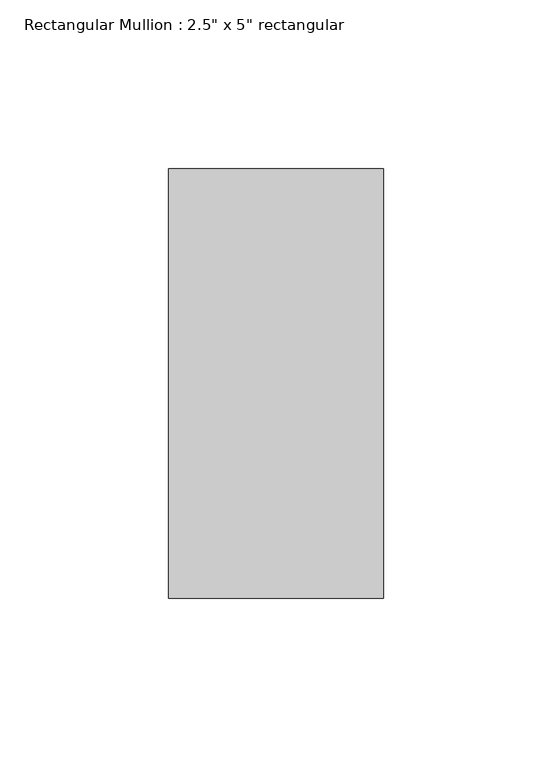
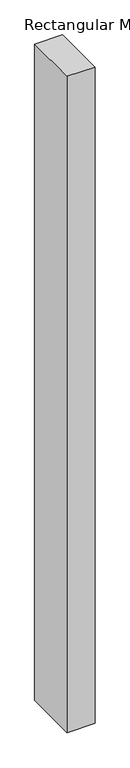
"""IFC4 building model written with IfcOpenShell, lengths in millimetres: member geometry."""

from ifc_helpers import new_model, si_unit, frame, origin, place, context, project, spatial, polyline, outline, extrude, source, transform, mapped, element, save


def member_7297827b(model_context):
    return source(origin(), model_context, "Body", "SweptSolid", [
        extrude(outline(polyline([(31.75, 63.5), (31.75, -63.5), (-31.75, -63.5), (-31.75, 63.5), (31.75, 63.5)])), frame((0.0, 0.0, -1571.0246189), z_axis=(0.0, 0.0, 1.0), x_axis=(1.0, 0.0, 0.0)), (0.0, 0.0, 1.0), 1571.0246189),
    ])


if __name__ == "__main__":
    model = new_model("IFC4")
    model_context = context("Model", 3, world=origin())
    ifc_project = project(units=[si_unit("LENGTHUNIT", "METRE", prefix="MILLI")], contexts=[model_context])
    site = spatial("IfcSite", under=ifc_project)
    building = spatial("IfcBuilding", under=site)
    placement = place(None, origin())
    member_shape = member_7297827b(model_context)
    element("IfcMember", 1, ObjectType="Rectangular Mullion : 2.5\" x 5\" rectangular", at=placement, inside=building, context=model_context, shape_type="MappedRepresentation", body=[
        mapped(member_shape, transform((0.0, 0.0, 0.0), x_axis=(1.0, 0.0, 0.0), y_axis=(0.0, 1.0, 0.0), z_axis=(0.0, 0.0, 1.0))),
    ])
    save(model, "model.ifc")

# Revit data of these elements
# Type "Rectangular Mullion : 2.5\" x 5\" rectangular"
#   built-in parameter 1007304 = 0.416667 (stored number, unit not read)
#   built-in parameter 1007301 = 0.104167 (stored number, unit not read)
#   built-in parameter 1007300 = 0.104167 (stored number, unit not read)
# Element 1 (IfcMember, "Rectangular Mullion : 2.5\" x 5\" rectangular")
#   Materials on its faces: "Aluminum"
# Materials
#   "Aluminum": class "Metal", colour RGB 247 247 247, transparency 0, Description = "Aluminum 6061", Cost = 0
